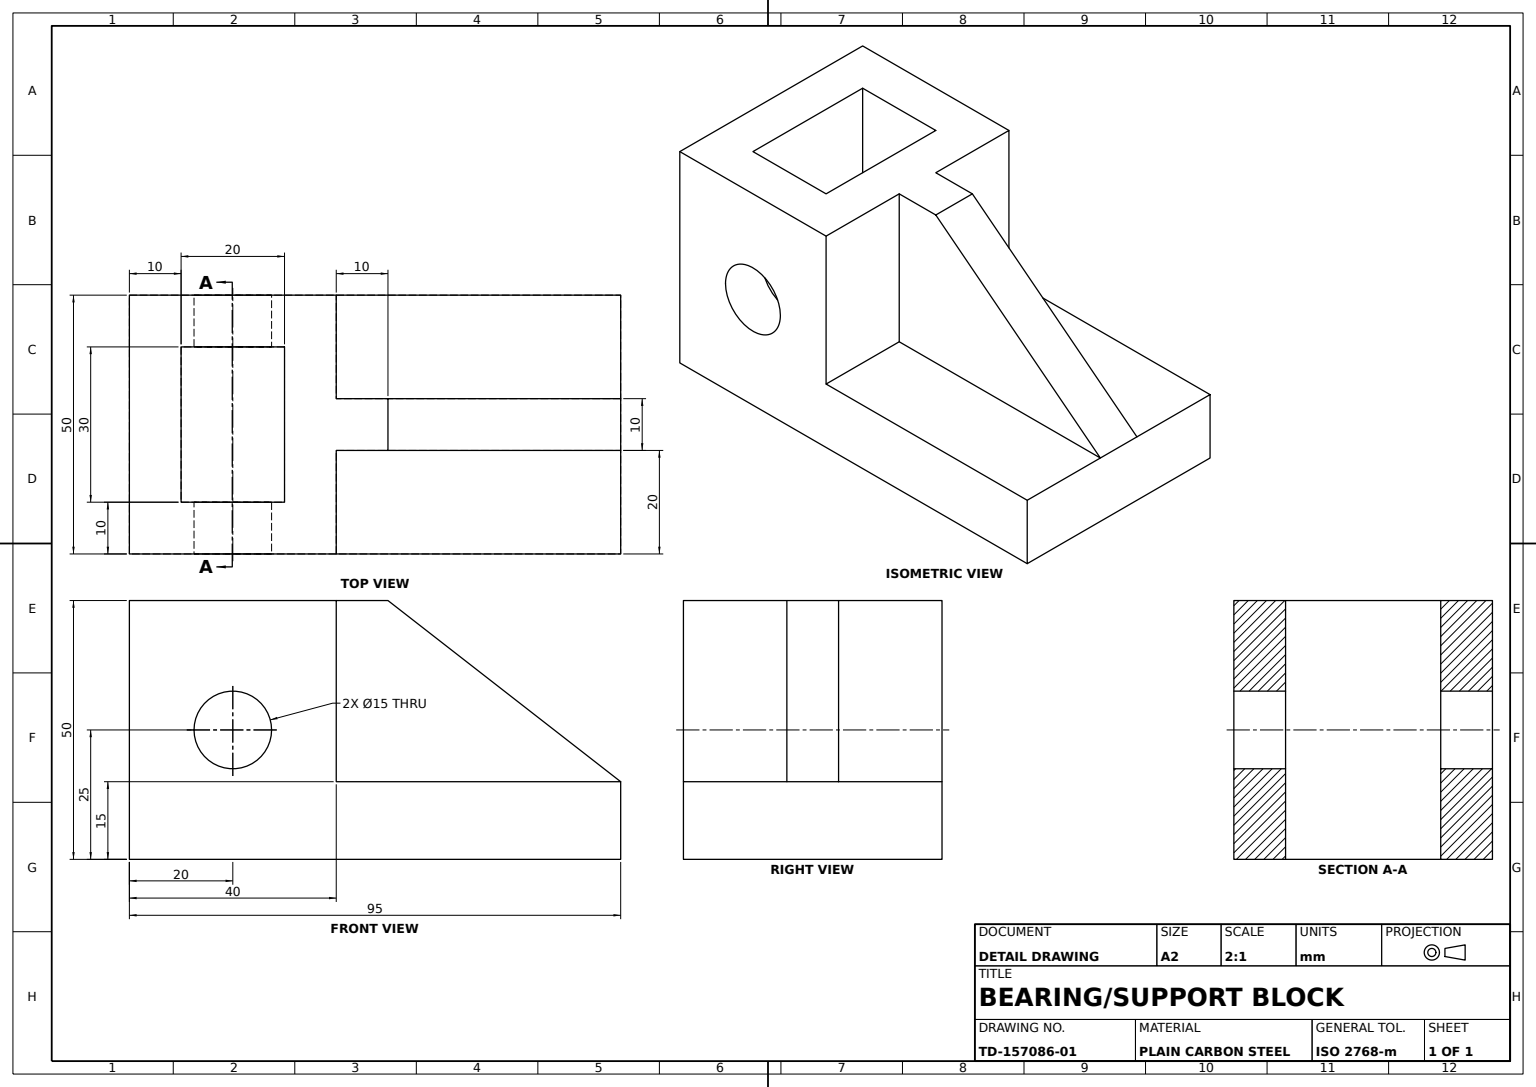
from build123d import *

# Parameters (mm, degrees)
BRACKET_BASE_50MM_DEPTH    = 50
HOLE_1_SKETCH_R            = 7.5
HOLE_1_CUT_10MM_DEEP_DEPTH = 10
HOLE_START                 = -10
HOLE_2_SKETCH_R            = 7.5
HOLE_2_CUT_10MM_DEEP_DEPTH = 10
RAISED_BOSS_SKETCH_W       = 10
RAISED_BOSS_SKETCH_H       = 10
RAISED_BOSS_35MM_DEPTH     = 35
GUSSET_RIB_10MM_REACH      = 112.227
GUSSET_RIB_SKETCH_WALL_W   = 279.462848106
GUSSET_RIB_SKETCH_WALL_H   = 10
SQUARE_POCKET_SKETCH_W     = 20
SQUARE_POCKET_SKETCH_H     = 30
SQUARE_POCKET_CUT_DEPTH    = 119.427192823


with BuildPart() as part:
    # Bracket Profile Sketch → Bracket Base 50mm (new body)
    with BuildSketch(Plane.XY):
        Polygon((0, 0), (95, 0), (95, 15), (40, 15), (40, 50), (0, 50), align=None)
    extrude(amount=BRACKET_BASE_50MM_DEPTH)

    # Hole 1 Sketch → Hole 1 Cut 10mm Deep (cut)
    with BuildSketch(Plane.XY.offset(50)):
        with Locations((20, 25)):
            Circle(HOLE_1_SKETCH_R)
    extrude(amount=-HOLE_1_CUT_10MM_DEEP_DEPTH, mode=Mode.SUBTRACT)

    # Hole 2 Sketch → Hole 2 Cut 10mm Deep (cut)
    with BuildSketch(Plane(origin=(0, 0, 0), x_dir=(-1, 0, 0), z_dir=(0, 0, -1)).offset(HOLE_START)):
        with Locations(Location((-20, 25, 0), (0, 0, 180))):
            Circle(HOLE_2_SKETCH_R)
    extrude(amount=HOLE_2_CUT_10MM_DEEP_DEPTH, mode=Mode.SUBTRACT)

    # Raised Boss Sketch → Raised Boss 35mm (add)
    with BuildSketch(Plane(origin=(0, 50, 0), x_dir=(1, 0, 0), z_dir=(0, 1, 0))):
        with Locations((45, -25)):
            Rectangle(RAISED_BOSS_SKETCH_W, RAISED_BOSS_SKETCH_H)
    extrude(amount=-RAISED_BOSS_35MM_DEPTH)

    # Gusset Rib Sketch wall → Gusset Rib 10mm (add, up to next)
    with BuildSketch(Plane(origin=(72.5, 32.5, 25), x_dir=(0.789352217376, -0.613940613515, 0), z_dir=(0.613940613515, 0.789352217376, 0)), mode=Mode.PRIVATE) as gusset_rib_10mm_sk1:
        Rectangle(GUSSET_RIB_SKETCH_WALL_W, GUSSET_RIB_SKETCH_WALL_H)
    gusset_rib_10mm_tool1 = extrude(gusset_rib_10mm_sk1.sketch, amount=-GUSSET_RIB_10MM_REACH, mode=Mode.PRIVATE) - part.part
    add(gusset_rib_10mm_tool1.solids().sort_by_distance((72.5, 32.5, 25))[0])

    # Square Pocket Sketch → Square Pocket Cut (cut, through all)
    with BuildSketch(Plane(origin=(0, 50, 0), x_dir=(1, 0, 0), z_dir=(0, 1, 0))):
        with Locations((20, -25)):
            Rectangle(SQUARE_POCKET_SKETCH_W, SQUARE_POCKET_SKETCH_H)
    extrude(amount=-SQUARE_POCKET_CUT_DEPTH, mode=Mode.SUBTRACT)


solid = part.part
